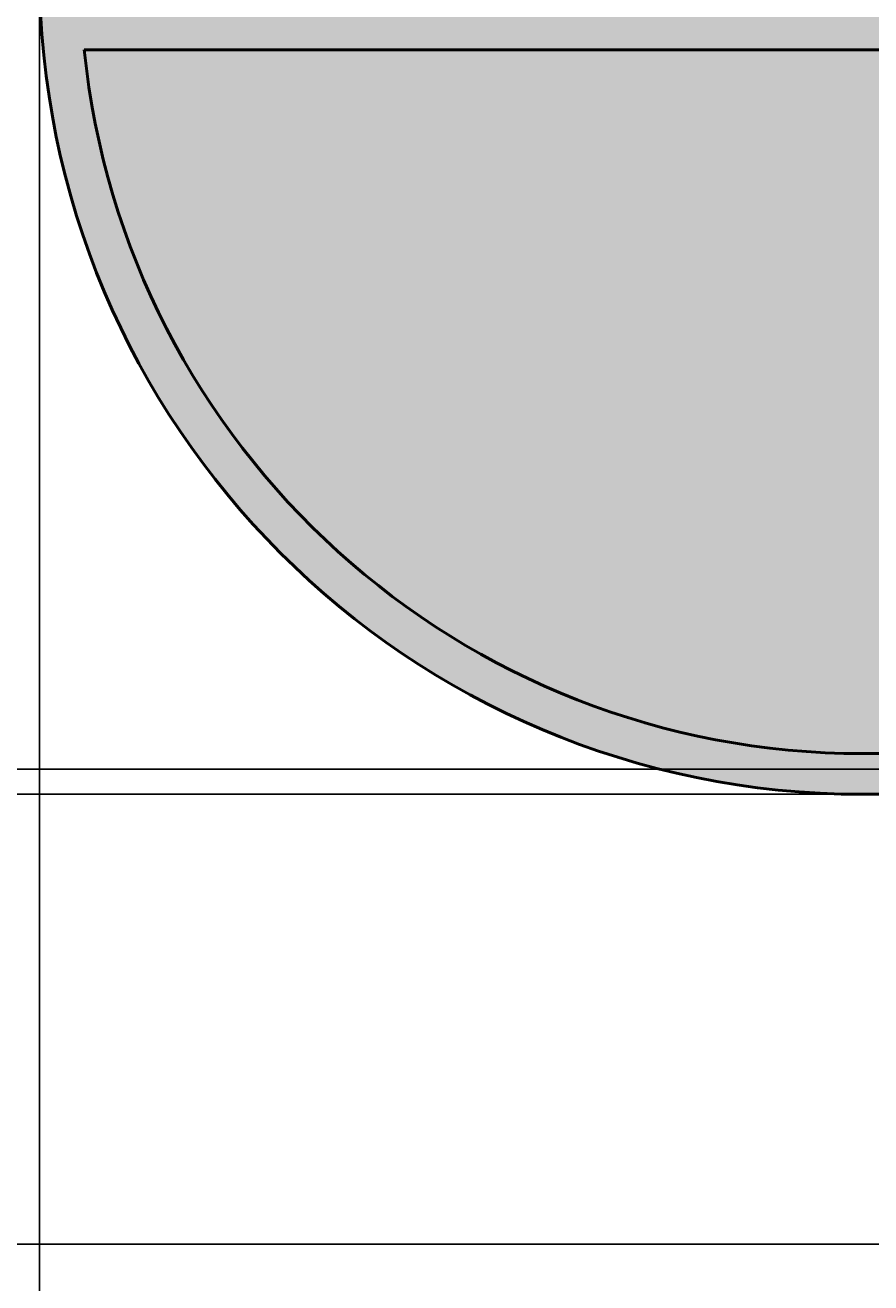
# Model space of a CAD drawing. Units: inches. Extents: x -12 to 334, y -10 to 186.
# Tile 4 of 77: x 3 to 24, y 49 to 79. Entities that reach past the tile are written whole.
import ezdxf

# ---------------------------------------------------------------- set-up
doc = ezdxf.new("R2010")
doc.units = ezdxf.units.IN
doc.header["$MEASUREMENT"] = 0
for name, color, linetype, lineweight in [('M-DIMS', 2, 'Continuous', 18), ('M-EQPM', 7, 'Continuous', 50), ('M-EQPM-PATT', 8, 'Continuous', 18)]:
    doc.layers.add(name, color=color, linetype=linetype, lineweight=lineweight)
doc.styles.get("Standard").update_dxf_attribs({"font": 'arial.ttf'})
doc.dimstyles.get("Standard").update_dxf_attribs({"dimtxt": 0.18, "dimasz": 0.18, "dimexe": 0.18, "dimexo": 0.0625, "dimgap": 0.09, "dimtad": 0, "dimtih": 1, "dimtoh": 1, "dimdec": 4, "dimzin": 0, "dimdsep": 46, "dimtxsty": 'Standard', "dimcen": 0.09, "dimadec": 0, "dimazin": 0, "dimtfac": 1, "dimtdec": 4, "dimtofl": 0, "dimtmove": 0, "dimatfit": 3, "dimfxl": 1, "dimtolj": 1, "dimtzin": 0, "dimarcsym": 0})

# ---------------------------------------------------------------- blocks, each defined once
blk = doc.blocks.new('*D1')
at = {"layer": 'Defpoints', "color": 0, "transparency": 16777216}
for p in [(281.426, 91.899), (3.376, 80.692), (281.426, 14.304)]:
    blk.add_point(p, dxfattribs=at)
at = {"layer": 'M-DIMS', "color": 0, "lineweight": -2, "transparency": 16777216}
for p, q in [((281.426, 91.836), (281.426, 14.124)), ((3.376, 80.629), (3.376, 14.124)), ((3.556, 14.304), (141.935, 14.304)), ((281.246, 14.304), (142.867, 14.304))]:
    blk.add_line(p, q, dxfattribs=at)
at = {"layer": 'M-DIMS', "color": 0, "transparency": 16777216}
for points in [[(3.556, 14.334), (3.556, 14.274), (3.376, 14.304)], [(281.246, 14.334), (281.246, 14.274), (281.426, 14.304)]]:
    blk.add_solid(points, dxfattribs=at)
at = {"layer": 'M-DIMS', "color": 0, "transparency": 16777216, "insert": (142.401, 14.304), "char_height": 0.18, "attachment_point": 5}
blk.add_mtext('\\A1;278.05', dxfattribs=at)
blk = doc.blocks.new('*D6')
at = {"layer": 'Defpoints', "color": 0, "transparency": 16777216}
for p in [(-11.174, 60.487), (23.581, 60.487), (32.1, 33.675)]:
    blk.add_point(p, dxfattribs=at)
at = {"layer": 'M-DIMS', "color": 0, "lineweight": -2, "transparency": 16777216}
for p, q in [((23.518, 60.487), (-11.354, 60.487)), ((-11.174, 60.307), (-11.174, 47.263)), ((-11.174, 33.855), (-11.174, 46.899)), ((32.038, 33.675), (-11.354, 33.675))]:
    blk.add_line(p, q, dxfattribs=at)
at = {"layer": 'M-DIMS', "color": 0, "transparency": 16777216}
for points in [[(-11.204, 60.307), (-11.144, 60.307), (-11.174, 60.487)], [(-11.204, 33.855), (-11.144, 33.855), (-11.174, 33.675)]]:
    blk.add_solid(points, dxfattribs=at)
at = {"layer": 'M-DIMS', "color": 0, "transparency": 16777216, "insert": (-11.174, 47.081), "char_height": 0.18, "attachment_point": 5}
blk.add_mtext('\\A1;26.81', dxfattribs=at)
blk = doc.blocks.new('*D7')
at = {"layer": 'Defpoints', "color": 0, "transparency": 16777216}
for p in [(-11.174, 100.896), (23.581, 100.896), (23.581, 60.487)]:
    blk.add_point(p, dxfattribs=at)
at = {"layer": 'M-DIMS', "color": 0, "lineweight": -2, "transparency": 16777216}
for p, q in [((23.518, 100.896), (-11.354, 100.896)), ((-11.174, 100.716), (-11.174, 80.873)), ((-11.174, 60.667), (-11.174, 80.51)), ((23.518, 60.487), (-11.354, 60.487))]:
    blk.add_line(p, q, dxfattribs=at)
at = {"layer": 'M-DIMS', "color": 0, "transparency": 16777216}
for points in [[(-11.204, 100.716), (-11.144, 100.716), (-11.174, 100.896)], [(-11.204, 60.667), (-11.144, 60.667), (-11.174, 60.487)]]:
    blk.add_solid(points, dxfattribs=at)
at = {"layer": 'M-DIMS', "color": 0, "transparency": 16777216, "insert": (-11.174, 80.692), "char_height": 0.18, "attachment_point": 5}
blk.add_mtext('\\A1;40.41', dxfattribs=at)
blk = doc.blocks.new('*D14')
at = {"layer": 'Defpoints', "color": 0, "transparency": 16777216}
for p in [(63.5, 109.058), (-11.174, 49.45), (64.207, 49.45)]:
    blk.add_point(p, dxfattribs=at)
at = {"layer": 'M-DIMS', "color": 0, "lineweight": -2, "transparency": 16777216}
for p, q in [((63.438, 109.058), (-11.354, 109.058)), ((-11.174, 108.878), (-11.174, 79.436)), ((-11.174, 49.63), (-11.174, 79.072)), ((64.144, 49.45), (-11.354, 49.45))]:
    blk.add_line(p, q, dxfattribs=at)
at = {"layer": 'M-DIMS', "color": 0, "transparency": 16777216}
for points in [[(-11.204, 108.878), (-11.144, 108.878), (-11.174, 109.058)], [(-11.204, 49.63), (-11.144, 49.63), (-11.174, 49.45)]]:
    blk.add_solid(points, dxfattribs=at)
at = {"layer": 'M-DIMS', "color": 0, "transparency": 16777216, "insert": (-11.174, 79.254), "char_height": 0.18, "attachment_point": 5}
blk.add_mtext('\\A1;59.61', dxfattribs=at)
blk = doc.blocks.new('*D35')
at = {"layer": 'Defpoints', "color": 0, "transparency": 16777216}
for p in [(216.428, 98.108), (-11.174, 61.105), (216.428, 61.105)]:
    blk.add_point(p, dxfattribs=at)
at = {"layer": 'M-DIMS', "color": 0, "lineweight": -2, "transparency": 16777216}
for p, q in [((216.365, 98.108), (-11.354, 98.108)), ((-11.174, 97.928), (-11.174, 79.788)), ((-11.174, 61.285), (-11.174, 79.424)), ((216.365, 61.105), (-11.354, 61.105))]:
    blk.add_line(p, q, dxfattribs=at)
at = {"layer": 'M-DIMS', "color": 0, "transparency": 16777216}
for points in [[(-11.204, 97.928), (-11.144, 97.928), (-11.174, 98.108)], [(-11.204, 61.285), (-11.144, 61.285), (-11.174, 61.105)]]:
    blk.add_solid(points, dxfattribs=at)
at = {"layer": 'M-DIMS', "color": 0, "transparency": 16777216, "insert": (-11.174, 79.606), "char_height": 0.18, "attachment_point": 5}
blk.add_mtext('\\A1;37', dxfattribs=at)
blk = doc.blocks.new('*D39')
at = {"layer": 'Defpoints', "color": 0, "transparency": 16777216}
for p in [(279.726, 80.692), (-11.174, 45.854), (269.381, 45.854)]:
    blk.add_point(p, dxfattribs=at)
at = {"layer": 'M-DIMS', "color": 0, "lineweight": -2, "transparency": 16777216}
for p, q in [((279.664, 80.692), (-11.354, 80.692)), ((-11.174, 80.512), (-11.174, 63.455)), ((-11.174, 46.034), (-11.174, 63.091)), ((269.318, 45.854), (-11.354, 45.854))]:
    blk.add_line(p, q, dxfattribs=at)
at = {"layer": 'M-DIMS', "color": 0, "transparency": 16777216}
for points in [[(-11.204, 80.512), (-11.144, 80.512), (-11.174, 80.692)], [(-11.204, 46.034), (-11.144, 46.034), (-11.174, 45.854)]]:
    blk.add_solid(points, dxfattribs=at)
at = {"layer": 'M-DIMS', "color": 0, "transparency": 16777216, "insert": (-11.174, 63.273), "char_height": 0.18, "attachment_point": 5}
blk.add_mtext('\\A1;34.84', dxfattribs=at)

msp = doc.modelspace()

# ---------------------------------------------------------------- hatches: boundary and pattern name
at = {"layer": 'M-EQPM-PATT'}
h = msp.add_hatch(color=256, dxfattribs=at)
h.set_gradient(color1=(99, 100, 102), color2=(99, 100, 102), tint=1)
h.paths.add_polyline_path([(4.3766, 80.754, -0.4132606), (23.5807, 99.8958), (37.1002, 99.8958), (37.1002, 127.7078), (32.1002, 127.7078), (32.1002, 125.2078), (36.1002, 125.2078), (36.1002, 100.8958), (23.5807, 100.8958, 1), (23.5807, 60.4872), (36.1002, 60.4872), (36.1002, 36.1752), (32.1002, 36.1752), (32.1002, 33.6752), (37.1002, 33.6752), (37.1002, 61.4872), (23.5807, 61.4872, -0.384914), (4.4744, 78.754), (72.9244, 78.754), (72.9244, 69.6117), (75.9244, 69.6117), (75.9244, 89.8963), (72.9244, 89.8963), (72.9244, 80.754)])
h.paths.add_polyline_path([(54.1002, 125.2078), (58.1002, 125.2078), (58.1002, 127.7078), (53.1002, 127.7078), (53.1002, 99.8958), (64.5, 99.8958), (64.5, 109.0583), (63.5, 109.0583), (63.5, 100.8958), (54.1002, 100.8958)], flags=17)
h.paths.add_polyline_path([(53.1002, 33.6752), (58.1002, 33.6752), (58.1002, 36.1752), (54.1002, 36.1752), (54.1002, 60.4872), (64.2068, 60.4872), (64.2068, 49.4497), (87.8879, 49.4497), (87.8879, 55.3205), (104.8919, 55.3205), (104.8919, 30.8541), (99.8919, 30.8541), (99.8919, 28.8541), (105.8919, 28.8541), (105.8919, 56.3205), (87.8879, 56.3205), (87.8879, 63.6117), (86.8879, 63.6117), (86.8879, 50.4497), (65.0061, 50.4497), (65.0061, 63.6117), (64.5, 63.6117), (64.5, 61.4872), (53.1002, 61.4872)])
h.paths.add_polyline_path([(121.8919, 28.8541), (121.8919, 30.8541), (116.8919, 30.8541), (116.8919, 45.8541), (209.6965, 45.8541), (209.9204, 46.8541), (115.8919, 46.8541), (115.8919, 28.8541)])
h.paths.add_polyline_path([(221.5761, 32.8541), (216.5761, 32.8541), (216.5761, 30.8541), (222.5761, 30.8541), (222.5761, 46.8541), (209.9204, 46.8541), (209.6965, 45.8541), (221.5761, 45.8541)])
h.paths.add_polyline_path([(233.5761, 45.8541), (249.8485, 45.8541), (249.3759, 46.8541), (232.5761, 46.8541), (232.5761, 30.8541), (238.5761, 30.8541), (238.5761, 32.8541), (233.5761, 32.8541)])
h = msp.add_hatch(color=256, dxfattribs=at)
h.set_gradient(color1=(205, 32, 39), color2=(205, 32, 39), tint=1)
h.paths.add_polyline_path([(64.5, 80.754), (64.5, 89.8963), (226.6083, 89.8963, -1), (226.6083, 69.6117), (64.5, 69.6117), (64.5, 78.754), (4.4744, 78.754, 0.384914), (23.5807, 61.4872), (37.1002, 61.4872), (37.1002, 33.6752), (53.1002, 33.6752), (53.1002, 61.4872), (64.5, 61.4872), (64.5, 63.6117), (226.6083, 63.6117, 1), (226.6083, 95.8963), (64.5, 95.8963), (64.5, 99.8958), (53.1002, 99.8958), (53.1002, 127.7078), (37.1002, 127.7078), (37.1002, 99.8958), (23.5807, 99.8958, 0.4132606), (4.3766, 80.754)])
h.paths.add_polyline_path([(64.5, 91.8963), (64.5, 93.8963), (226.6083, 93.8963, -1), (226.6083, 65.6117), (64.5, 65.6117), (64.5, 67.6117), (226.6083, 67.6117, 1), (226.6083, 91.8963)], flags=16)

# ---------------------------------------------------------------- linework, layer by layer
at = {"layer": 'M-EQPM'}
msp.add_line((72.9244, 78.754), (4.4744, 78.754), dxfattribs=at)
for points in [[(36.1002, 60.4872), (23.5807, 60.4872, -1), (23.5807, 100.8958), (36.1002, 100.8958)], [(37.1002, 61.4872), (23.5807, 61.4872, -0.384914), (4.4744, 78.754, -0.384914)]]:
    msp.add_lwpolyline(points, format="xyb", dxfattribs=at)

# ---------------------------------------------------------------- dimensions: what is measured, and where the dimension line sits
at = {"layer": 'M-DIMS'}
for base, p1, p2, override, picture, middle in [((-11.1736, 49.4497), (63.5, 109.0583), (64.2068, 49.4497), {"dimdec": 2, "dimlfac": 1, "dimrnd": 0, "dimzin": 0, "dimdsep": 46, "dimlunit": 2}, '*D14', (-11.1735, 79.254)), ((-11.1736, 100.8958), (23.5807, 60.4872), (23.5807, 100.8958), {"dimdec": 2, "dimlfac": 1, "dimrnd": 0, "dimzin": 0, "dimdsep": 46, "dimlunit": 2}, '*D7', (-11.1735, 80.6915)), ((-11.1736, 61.1045), (216.4278, 98.1081), (216.4278, 61.1045), {"dimdec": 0, "dimlfac": 1, "dimrnd": 0, "dimzin": 0, "dimdsep": 46, "dimlunit": 2}, '*D35', (-11.1735, 79.6063)), ((-11.1736, 45.8541), (279.7263, 80.6915), (269.3808, 45.8541), {"dimdec": 2, "dimlfac": 1, "dimrnd": 0, "dimzin": 0, "dimdsep": 46, "dimlunit": 2}, '*D39', (-11.1735, 63.2728)), ((-11.1736, 60.4872), (32.1002, 33.6752), (23.5807, 60.4872), {"dimdec": 2, "dimlfac": 1, "dimrnd": 0, "dimzin": 0, "dimdsep": 46, "dimlunit": 2}, '*D6', (-11.1735, 47.0812))]:
    dim = msp.add_linear_dim(base=base, p1=p1, p2=p2, angle=90, dimstyle='Standard', override=override, dxfattribs=at)
    dim.commit()
    dim.dimension.update_dxf_attribs({"geometry": picture, "text_midpoint": middle})
dim = msp.add_linear_dim(base=(281.4256, 14.3041), p1=(3.3765, 80.6915), p2=(281.4256, 91.8988), dimstyle='Standard', override={"dimdec": 2, "dimlfac": 1, "dimrnd": 0, "dimzin": 0, "dimdsep": 46, "dimlunit": 2}, dxfattribs=at)
dim.commit()
dim.dimension.update_dxf_attribs({"geometry": '*D1', "text_midpoint": (142.401, 14.3041)})

doc.saveas('drawing.dxf')
